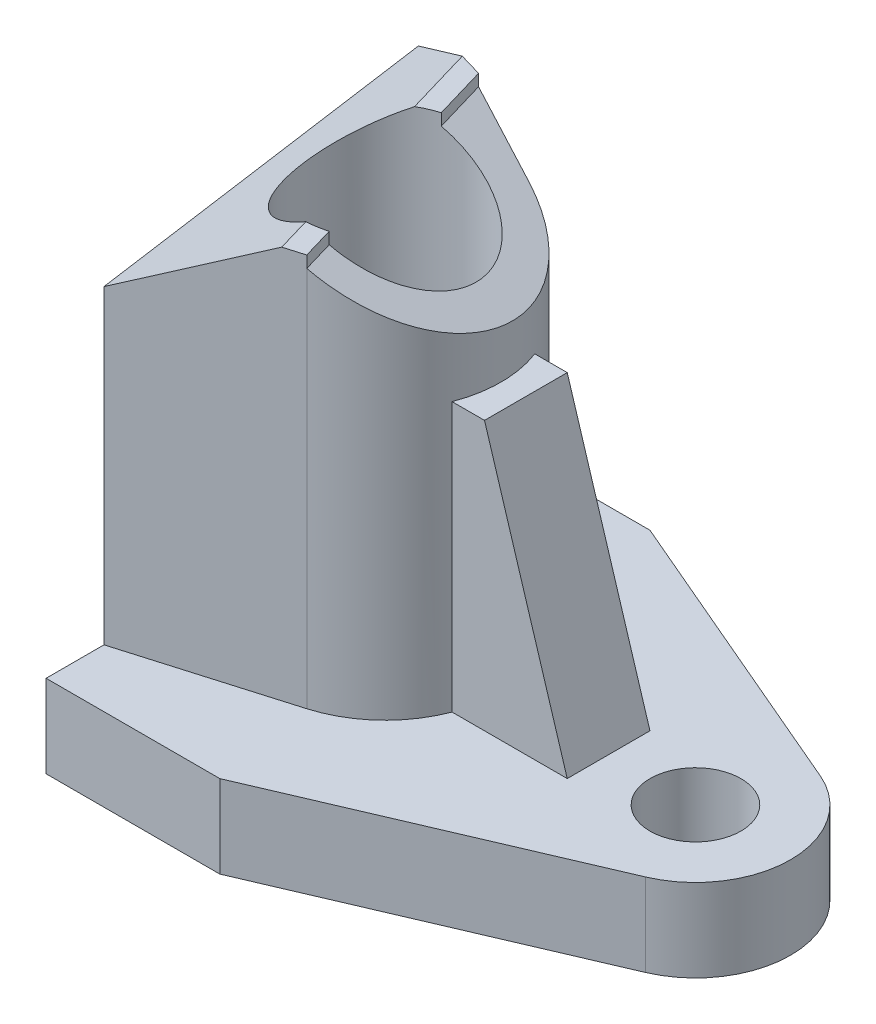
ISO-10303-21;
HEADER;
FILE_DESCRIPTION(('STEP AP214'),'2;1');
FILE_NAME('part.step','',(''),(''),'','','');
FILE_SCHEMA(('AUTOMOTIVE_DESIGN { 1 0 10303 214 1 1 1 1 }'));
ENDSEC;
DATA;
#1=APPLICATION_CONTEXT('core data for automotive mechanical design processes');
#2=APPLICATION_PROTOCOL_DEFINITION('international standard','automotive_design',2000,#1);
#3=PRODUCT_CONTEXT('',#1,'mechanical');
#4=PRODUCT('Part','Part','',(#3));
#5=PRODUCT_RELATED_PRODUCT_CATEGORY('part','',(#4));
#6=PRODUCT_DEFINITION_FORMATION('','',#4);
#7=PRODUCT_DEFINITION_CONTEXT('part definition',#1,'design');
#8=PRODUCT_DEFINITION('design','',#6,#7);
#9=PRODUCT_DEFINITION_SHAPE('','',#8);
#10=(LENGTH_UNIT() NAMED_UNIT(*) SI_UNIT(.MILLI.,.METRE.));
#11=(NAMED_UNIT(*) PLANE_ANGLE_UNIT() SI_UNIT($,.RADIAN.));
#12=(NAMED_UNIT(*) SI_UNIT($,.STERADIAN.) SOLID_ANGLE_UNIT());
#13=UNCERTAINTY_MEASURE_WITH_UNIT(LENGTH_MEASURE(1.E-05),#10,'distance_accuracy_value','');
#14=(GEOMETRIC_REPRESENTATION_CONTEXT(3) GLOBAL_UNCERTAINTY_ASSIGNED_CONTEXT((#13)) GLOBAL_UNIT_ASSIGNED_CONTEXT((#10,
#11,#12)) REPRESENTATION_CONTEXT('',''));
#15=CARTESIAN_POINT('',(0.,0.,0.));
#16=DIRECTION('',(0.,0.,1.));
#17=DIRECTION('',(1.,0.,0.));
#18=AXIS2_PLACEMENT_3D('',#15,#16,#17);
#19=CARTESIAN_POINT('',(-21.,10.,0.));
#20=DIRECTION('',(-1.,0.,0.));
#21=DIRECTION('',(0.,0.,1.));
#22=AXIS2_PLACEMENT_3D('',#19,#20,#21);
#23=PLANE('',#22);
#24=DIRECTION('',(0.,-1.,0.));
#25=VECTOR('',#24,1.);
#26=CARTESIAN_POINT('',(-21.,10.,-26.));
#27=LINE('',#26,#25);
#28=CARTESIAN_POINT('',(-21.,10.,-26.));
#29=VERTEX_POINT('',#28);
#30=CARTESIAN_POINT('',(-21.,0.,-26.));
#31=VERTEX_POINT('',#30);
#32=EDGE_CURVE('E290',#29,#31,#27,.T.);
#33=ORIENTED_EDGE('',*,*,#32,.T.);
#34=DIRECTION('',(0.,0.,-1.));
#35=VECTOR('',#34,1.);
#36=CARTESIAN_POINT('',(-21.,0.,0.));
#37=LINE('',#36,#35);
#38=CARTESIAN_POINT('',(-21.,0.,26.));
#39=VERTEX_POINT('',#38);
#40=EDGE_CURVE('E271',#39,#31,#37,.T.);
#41=ORIENTED_EDGE('',*,*,#40,.F.);
#42=DIRECTION('',(0.,-1.,0.));
#43=VECTOR('',#42,1.);
#44=CARTESIAN_POINT('',(-21.,10.,26.));
#45=LINE('',#44,#43);
#46=CARTESIAN_POINT('',(-21.,10.,26.));
#47=VERTEX_POINT('',#46);
#48=EDGE_CURVE('E312',#47,#39,#45,.T.);
#49=ORIENTED_EDGE('',*,*,#48,.F.);
#50=DIRECTION('',(0.,0.,-1.));
#51=VECTOR('',#50,1.);
#52=CARTESIAN_POINT('',(-21.,10.,0.));
#53=LINE('',#52,#51);
#54=CARTESIAN_POINT('',(-21.,10.,19.));
#55=VERTEX_POINT('',#54);
#56=EDGE_CURVE('E275',#47,#55,#53,.T.);
#57=ORIENTED_EDGE('',*,*,#56,.T.);
#58=DIRECTION('',(0.,-1.,0.));
#59=VECTOR('',#58,1.);
#60=CARTESIAN_POINT('',(-21.,57.5,19.));
#61=LINE('',#60,#59);
#62=CARTESIAN_POINT('',(-21.,47.5055162672704,19.));
#63=VERTEX_POINT('',#62);
#64=EDGE_CURVE('E252',#63,#55,#61,.T.);
#65=ORIENTED_EDGE('',*,*,#64,.F.);
#66=DIRECTION('',(0.,0.160666455096198,-0.987008758931156));
#67=VECTOR('',#66,1.);
#68=CARTESIAN_POINT('',(-21.,49.5503645251847,6.4380551930513));
#69=LINE('',#68,#67);
#70=CARTESIAN_POINT('',(-21.,53.6912012861827,-19.0000000000011));
#71=VERTEX_POINT('',#70);
#72=EDGE_CURVE('E231',#63,#71,#69,.T.);
#73=ORIENTED_EDGE('',*,*,#72,.T.);
#74=DIRECTION('',(0.,-1.,0.));
#75=VECTOR('',#74,1.);
#76=CARTESIAN_POINT('',(-21.,57.5,-19.0000000000011));
#77=LINE('',#76,#75);
#78=CARTESIAN_POINT('',(-21.,10.,-19.0000000000011));
#79=VERTEX_POINT('',#78);
#80=EDGE_CURVE('E265',#71,#79,#77,.T.);
#81=ORIENTED_EDGE('',*,*,#80,.T.);
#82=EDGE_CURVE('E277',#79,#29,#53,.T.);
#83=ORIENTED_EDGE('',*,*,#82,.T.);
#84=EDGE_LOOP('',(#33,#41,#49,#57,#65,#73,#81,#83));
#85=FACE_BOUND('',#84,.T.);
#86=ADVANCED_FACE('F45',(#85),#23,.T.);
#87=CARTESIAN_POINT('',(3.4702751003222,57.5,11.8089854095073));
#88=DIRECTION('',(-0.281945282430885,0.,-0.959430486129646));
#89=DIRECTION('',(-0.959430486129646,0.,0.281945282430885));
#90=AXIS2_PLACEMENT_3D('',#87,#88,#89);
#91=PLANE('',#90);
#92=DIRECTION('',(-0.83089117415353,-0.499999999999995,0.244171777062326));
#93=VECTOR('',#92,1.);
#94=CARTESIAN_POINT('',(-22.383250769799,46.6731264111571,19.4064922207517));
#95=LINE('',#94,#93);
#96=CARTESIAN_POINT('',(-4.39134335250773,57.5,14.1192582923178));
#97=VERTEX_POINT('',#96);
#98=EDGE_CURVE('E209',#97,#63,#95,.T.);
#99=ORIENTED_EDGE('',*,*,#98,.T.);
#100=ORIENTED_EDGE('',*,*,#64,.T.);
#101=DIRECTION('',(0.959430486129646,0.,-0.281945282430885));
#102=VECTOR('',#101,1.);
#103=CARTESIAN_POINT('',(3.4702751003222,10.,11.8089854095073));
#104=LINE('',#103,#102);
#105=CARTESIAN_POINT('',(-2.05276604596761,10.,13.432026805815));
#106=VERTEX_POINT('',#105);
#107=EDGE_CURVE('E243',#55,#106,#104,.T.);
#108=ORIENTED_EDGE('',*,*,#107,.T.);
#109=DIRECTION('',(0.,-1.,0.));
#110=VECTOR('',#109,1.);
#111=CARTESIAN_POINT('',(-2.05276604596761,57.5,13.432026805815));
#112=LINE('',#111,#110);
#113=CARTESIAN_POINT('',(-2.05276604596761,56.0927294817384,13.432026805815));
#114=VERTEX_POINT('',#113);
#115=EDGE_CURVE('E270',#114,#106,#112,.T.);
#116=ORIENTED_EDGE('',*,*,#115,.F.);
#117=CARTESIAN_POINT('',(-2.05276604596762,57.5,13.432026805815));
#118=VERTEX_POINT('',#117);
#119=EDGE_CURVE('E268',#118,#114,#112,.T.);
#120=ORIENTED_EDGE('',*,*,#119,.F.);
#121=DIRECTION('',(0.959430486129646,0.,-0.281945282430885));
#122=VECTOR('',#121,1.);
#123=CARTESIAN_POINT('',(3.4702751003222,57.5,11.8089854095073));
#124=LINE('',#123,#122);
#125=EDGE_CURVE('E242',#97,#118,#124,.T.);
#126=ORIENTED_EDGE('',*,*,#125,.F.);
#127=EDGE_LOOP('',(#99,#100,#108,#116,#120,#126));
#128=FACE_BOUND('',#127,.T.);
#129=ADVANCED_FACE('F341',(#128),#91,.F.);
#130=CARTESIAN_POINT('',(3.47027510032275,57.5,-11.8089854095068));
#131=DIRECTION('',(0.281945282430936,0.,-0.959430486129631));
#132=DIRECTION('',(-0.959430486129631,0.,-0.281945282430936));
#133=AXIS2_PLACEMENT_3D('',#130,#131,#132);
#134=PLANE('',#133);
#135=ORIENTED_EDGE('',*,*,#80,.F.);
#136=DIRECTION('',(0.863068045718996,0.436791294924048,0.253627508636911));
#137=VECTOR('',#136,1.);
#138=CARTESIAN_POINT('',(0.23751690836758,64.4393254432408,-12.7589874520087));
#139=LINE('',#138,#137);
#140=CARTESIAN_POINT('',(-13.4740888825568,57.5,-16.788380538004));
#141=VERTEX_POINT('',#140);
#142=EDGE_CURVE('E232',#71,#141,#139,.T.);
#143=ORIENTED_EDGE('',*,*,#142,.T.);
#144=DIRECTION('',(0.959430486129631,0.,0.281945282430936));
#145=VECTOR('',#144,1.);
#146=CARTESIAN_POINT('',(3.47027510032275,57.5,-11.8089854095068));
#147=LINE('',#146,#145);
#148=CARTESIAN_POINT('',(-10.6934239972705,57.5,-15.9712339518136));
#149=VERTEX_POINT('',#148);
#150=EDGE_CURVE('E250',#141,#149,#147,.T.);
#151=ORIENTED_EDGE('',*,*,#150,.T.);
#152=DIRECTION('',(0.,-1.,0.));
#153=VECTOR('',#152,1.);
#154=CARTESIAN_POINT('',(-10.6934239972705,57.5,-15.9712339518136));
#155=LINE('',#154,#153);
#156=CARTESIAN_POINT('',(-10.6934239972705,56.0927294817384,-15.9712339518136));
#157=VERTEX_POINT('',#156);
#158=EDGE_CURVE('E221',#149,#157,#155,.T.);
#159=ORIENTED_EDGE('',*,*,#158,.T.);
#160=DIRECTION('',(-0.863068045718993,0.436791294924054,-0.25362750863691));
#161=VECTOR('',#160,1.);
#162=CARTESIAN_POINT('',(0.237516908367499,50.5606745567591,-12.7589874520087));
#163=LINE('',#162,#161);
#164=CARTESIAN_POINT('',(-2.05276604596688,51.7197670087718,-13.4320268058148));
#165=VERTEX_POINT('',#164);
#166=EDGE_CURVE('E230',#165,#157,#163,.T.);
#167=ORIENTED_EDGE('',*,*,#166,.F.);
#168=DIRECTION('',(0.,-1.,0.));
#169=VECTOR('',#168,1.);
#170=CARTESIAN_POINT('',(-2.05276604596688,57.5,-13.4320268058148));
#171=LINE('',#170,#169);
#172=CARTESIAN_POINT('',(-2.05276604596688,10.,-13.4320268058148));
#173=VERTEX_POINT('',#172);
#174=EDGE_CURVE('E262',#165,#173,#171,.T.);
#175=ORIENTED_EDGE('',*,*,#174,.T.);
#176=DIRECTION('',(0.959430486129631,0.,0.281945282430936));
#177=VECTOR('',#176,1.);
#178=CARTESIAN_POINT('',(3.47027510032275,10.,-11.8089854095068));
#179=LINE('',#178,#177);
#180=EDGE_CURVE('E246',#79,#173,#179,.T.);
#181=ORIENTED_EDGE('',*,*,#180,.F.);
#182=EDGE_LOOP('',(#135,#143,#151,#159,#167,#175,#181));
#183=FACE_BOUND('',#182,.T.);
#184=ADVANCED_FACE('F348',(#183),#134,.T.);
#185=CARTESIAN_POINT('',(0.,57.5,0.));
#186=DIRECTION('',(0.,1.,0.));
#187=DIRECTION('',(0.,0.,1.));
#188=AXIS2_PLACEMENT_3D('',#185,#186,#187);
#189=PLANE('',#188);
#190=ORIENTED_EDGE('',*,*,#150,.F.);
#191=DIRECTION('',(0.281945282430885,0.,0.959430486129646));
#192=VECTOR('',#191,1.);
#193=CARTESIAN_POINT('',(-17.7837442679748,57.5,-31.4536897988404));
#194=LINE('',#193,#192);
#195=CARTESIAN_POINT('',(-11.0729926210932,57.5,-8.61769956927799));
#196=VERTEX_POINT('',#195);
#197=EDGE_CURVE('E216',#141,#196,#194,.T.);
#198=ORIENTED_EDGE('',*,*,#197,.T.);
#199=CARTESIAN_POINT('',(-6.,57.5,0.));
#200=DIRECTION('',(0.,1.,0.));
#201=DIRECTION('',(0.,0.,1.));
#202=AXIS2_PLACEMENT_3D('',#199,#200,#201);
#203=CIRCLE('',#202,10.);
#204=CARTESIAN_POINT('',(-8.81945282430885,57.5,-9.59430486129646));
#205=VERTEX_POINT('',#204);
#206=EDGE_CURVE('E240',#205,#196,#203,.T.);
#207=ORIENTED_EDGE('',*,*,#206,.F.);
#208=DIRECTION('',(0.281945282430885,0.,0.959430486129646));
#209=VECTOR('',#208,1.);
#210=CARTESIAN_POINT('',(-15.4451669614347,57.5,-32.1409212853431));
#211=LINE('',#210,#209);
#212=EDGE_CURVE('E222',#149,#205,#211,.T.);
#213=ORIENTED_EDGE('',*,*,#212,.F.);
#214=EDGE_LOOP('',(#190,#198,#207,#213));
#215=FACE_BOUND('',#214,.T.);
#216=ADVANCED_FACE('F396',(#215),#189,.T.);
#217=CARTESIAN_POINT('',(-5.60416199198704,57.5,9.99216254228345));
#218=VERTEX_POINT('',#217);
#219=CARTESIAN_POINT('',(-3.18054717569115,57.5,9.59430486129646));
#220=VERTEX_POINT('',#219);
#221=EDGE_CURVE('E245',#218,#220,#203,.T.);
#222=ORIENTED_EDGE('',*,*,#221,.F.);
#223=EDGE_CURVE('E213',#218,#97,#194,.T.);
#224=ORIENTED_EDGE('',*,*,#223,.T.);
#225=ORIENTED_EDGE('',*,*,#125,.T.);
#226=EDGE_CURVE('E225',#220,#118,#211,.T.);
#227=ORIENTED_EDGE('',*,*,#226,.F.);
#228=EDGE_LOOP('',(#222,#224,#225,#227));
#229=FACE_BOUND('',#228,.T.);
#230=ADVANCED_FACE('F389',(#229),#189,.T.);
#231=CARTESIAN_POINT('',(-6.,10.,0.));
#232=DIRECTION('',(0.,1.,0.));
#233=DIRECTION('',(0.,0.,1.));
#234=AXIS2_PLACEMENT_3D('',#231,#232,#233);
#235=CYLINDRICAL_SURFACE('',#234,10.);
#236=CARTESIAN_POINT('',(-6.,10.,0.));
#237=DIRECTION('',(0.,1.,0.));
#238=DIRECTION('',(0.,0.,1.));
#239=AXIS2_PLACEMENT_3D('',#236,#237,#238);
#240=CIRCLE('',#239,10.);
#241=CARTESIAN_POINT('',(-6.,10.,10.));
#242=VERTEX_POINT('',#241);
#243=EDGE_CURVE('E236',#242,#242,#240,.T.);
#244=ORIENTED_EDGE('',*,*,#243,.F.);
#245=EDGE_LOOP('',(#244));
#246=FACE_BOUND('',#245,.T.);
#247=CARTESIAN_POINT('',(-6.,58.9072705182616,0.));
#248=DIRECTION('',(-0.479715243064818,0.866025403784442,0.140972641215441));
#249=DIRECTION('',(0.83089117415353,0.499999999999995,-0.244171777062326));
#250=AXIS2_PLACEMENT_3D('',#247,#248,#249);
#251=ELLIPSE('',#250,11.5470053837925,10.);
#252=EDGE_CURVE('E47',#218,#196,#251,.F.);
#253=ORIENTED_EDGE('',*,*,#252,.F.);
#254=ORIENTED_EDGE('',*,*,#221,.T.);
#255=DIRECTION('',(0.,1.,0.));
#256=VECTOR('',#255,1.);
#257=CARTESIAN_POINT('',(-3.18054717569115,10.,9.59430486129646));
#258=LINE('',#257,#256);
#259=CARTESIAN_POINT('',(-3.18054717569115,56.0927294817384,9.59430486129646));
#260=VERTEX_POINT('',#259);
#261=EDGE_CURVE('E320',#260,#220,#258,.T.);
#262=ORIENTED_EDGE('',*,*,#261,.F.);
#263=CARTESIAN_POINT('',(-6.,56.0927294817384,0.));
#264=DIRECTION('',(-0.479715243064824,-0.866025403784438,0.140972641215443));
#265=DIRECTION('',(-0.830891174153526,0.500000000000001,0.244171777062325));
#266=AXIS2_PLACEMENT_3D('',#263,#264,#265);
#267=ELLIPSE('',#266,11.5470053837925,10.);
#268=CARTESIAN_POINT('',(-8.81945282430885,56.0927294817384,-9.59430486129646));
#269=VERTEX_POINT('',#268);
#270=EDGE_CURVE('E317',#260,#269,#267,.F.);
#271=ORIENTED_EDGE('',*,*,#270,.T.);
#272=DIRECTION('',(0.,1.,0.));
#273=VECTOR('',#272,1.);
#274=CARTESIAN_POINT('',(-8.81945282430885,10.,-9.59430486129646));
#275=LINE('',#274,#273);
#276=EDGE_CURVE('E325',#205,#269,#275,.F.);
#277=ORIENTED_EDGE('',*,*,#276,.F.);
#278=ORIENTED_EDGE('',*,*,#206,.T.);
#279=EDGE_LOOP('',(#253,#254,#262,#271,#277,#278));
#280=FACE_BOUND('',#279,.T.);
#281=ADVANCED_FACE('F395',(#246,#280),#235,.F.);
#282=CARTESIAN_POINT('',(0.,10.,26.));
#283=DIRECTION('',(0.,0.,-1.));
#284=DIRECTION('',(-1.,0.,0.));
#285=AXIS2_PLACEMENT_3D('',#282,#283,#284);
#286=PLANE('',#285);
#287=DIRECTION('',(1.,0.,0.));
#288=VECTOR('',#287,1.);
#289=CARTESIAN_POINT('',(0.,0.,26.));
#290=LINE('',#289,#288);
#291=CARTESIAN_POINT('',(0.,0.,26.));
#292=VERTEX_POINT('',#291);
#293=EDGE_CURVE('E288',#39,#292,#290,.T.);
#294=ORIENTED_EDGE('',*,*,#293,.T.);
#295=DIRECTION('',(0.,-1.,0.));
#296=VECTOR('',#295,1.);
#297=CARTESIAN_POINT('',(0.,10.,26.));
#298=LINE('',#297,#296);
#299=CARTESIAN_POINT('',(0.,10.,26.));
#300=VERTEX_POINT('',#299);
#301=EDGE_CURVE('E315',#300,#292,#298,.T.);
#302=ORIENTED_EDGE('',*,*,#301,.F.);
#303=DIRECTION('',(1.,0.,0.));
#304=VECTOR('',#303,1.);
#305=CARTESIAN_POINT('',(0.,10.,26.));
#306=LINE('',#305,#304);
#307=EDGE_CURVE('E274',#47,#300,#306,.T.);
#308=ORIENTED_EDGE('',*,*,#307,.F.);
#309=ORIENTED_EDGE('',*,*,#48,.T.);
#310=EDGE_LOOP('',(#294,#302,#308,#309));
#311=FACE_BOUND('',#310,.T.);
#312=ADVANCED_FACE('F368',(#311),#286,.F.);
#313=CARTESIAN_POINT('',(9.40890232991811,10.,21.9706497504953));
#314=DIRECTION('',(-0.393668654576833,0.,-0.919252408429625));
#315=DIRECTION('',(-0.919252408429625,0.,0.393668654576833));
#316=AXIS2_PLACEMENT_3D('',#313,#314,#315);
#317=PLANE('',#316);
#318=DIRECTION('',(0.919252408429625,0.,-0.393668654576833));
#319=VECTOR('',#318,1.);
#320=CARTESIAN_POINT('',(9.40890232991811,0.,21.9706497504953));
#321=LINE('',#320,#319);
#322=CARTESIAN_POINT('',(36.0271895276336,0.,10.5714026969407));
#323=VERTEX_POINT('',#322);
#324=EDGE_CURVE('E295',#292,#323,#321,.T.);
#325=ORIENTED_EDGE('',*,*,#324,.T.);
#326=DIRECTION('',(0.,-1.,0.));
#327=VECTOR('',#326,1.);
#328=CARTESIAN_POINT('',(36.0271895276336,10.,10.5714026969407));
#329=LINE('',#328,#327);
#330=CARTESIAN_POINT('',(36.0271895276336,10.,10.5714026969407));
#331=VERTEX_POINT('',#330);
#332=EDGE_CURVE('E310',#331,#323,#329,.T.);
#333=ORIENTED_EDGE('',*,*,#332,.F.);
#334=DIRECTION('',(0.919252408429625,0.,-0.393668654576833));
#335=VECTOR('',#334,1.);
#336=CARTESIAN_POINT('',(9.40890232991811,10.,21.9706497504953));
#337=LINE('',#336,#335);
#338=EDGE_CURVE('E279',#300,#331,#337,.T.);
#339=ORIENTED_EDGE('',*,*,#338,.F.);
#340=ORIENTED_EDGE('',*,*,#301,.T.);
#341=EDGE_LOOP('',(#325,#333,#339,#340));
#342=FACE_BOUND('',#341,.T.);
#343=ADVANCED_FACE('F367',(#342),#317,.F.);
#344=CARTESIAN_POINT('',(31.5,10.,0.));
#345=DIRECTION('',(0.,-1.,0.));
#346=DIRECTION('',(0.,0.,-1.));
#347=AXIS2_PLACEMENT_3D('',#344,#345,#346);
#348=CYLINDRICAL_SURFACE('',#347,11.5);
#349=CARTESIAN_POINT('',(31.5,0.,0.));
#350=DIRECTION('',(0.,1.,0.));
#351=DIRECTION('',(0.,0.,1.));
#352=AXIS2_PLACEMENT_3D('',#349,#350,#351);
#353=CIRCLE('',#352,11.5);
#354=CARTESIAN_POINT('',(36.0271895276336,0.,-10.5714026969407));
#355=VERTEX_POINT('',#354);
#356=EDGE_CURVE('E294',#323,#355,#353,.T.);
#357=ORIENTED_EDGE('',*,*,#356,.T.);
#358=DIRECTION('',(0.,-1.,0.));
#359=VECTOR('',#358,1.);
#360=CARTESIAN_POINT('',(36.0271895276336,10.,-10.5714026969407));
#361=LINE('',#360,#359);
#362=CARTESIAN_POINT('',(36.0271895276336,10.,-10.5714026969407));
#363=VERTEX_POINT('',#362);
#364=EDGE_CURVE('E307',#363,#355,#361,.T.);
#365=ORIENTED_EDGE('',*,*,#364,.F.);
#366=CARTESIAN_POINT('',(31.5,10.,0.));
#367=DIRECTION('',(0.,1.,0.));
#368=DIRECTION('',(0.,0.,1.));
#369=AXIS2_PLACEMENT_3D('',#366,#367,#368);
#370=CIRCLE('',#369,11.5);
#371=EDGE_CURVE('E278',#331,#363,#370,.T.);
#372=ORIENTED_EDGE('',*,*,#371,.F.);
#373=ORIENTED_EDGE('',*,*,#332,.T.);
#374=EDGE_LOOP('',(#357,#365,#372,#373));
#375=FACE_BOUND('',#374,.T.);
#376=ADVANCED_FACE('F410',(#375),#348,.T.);
#377=CARTESIAN_POINT('',(9.4089023299181,10.,-21.9706497504953));
#378=DIRECTION('',(0.393668654576833,0.,-0.919252408429625));
#379=DIRECTION('',(-0.919252408429625,0.,-0.393668654576833));
#380=AXIS2_PLACEMENT_3D('',#377,#378,#379);
#381=PLANE('',#380);
#382=DIRECTION('',(0.919252408429625,0.,0.393668654576833));
#383=VECTOR('',#382,1.);
#384=CARTESIAN_POINT('',(9.4089023299181,0.,-21.9706497504953));
#385=LINE('',#384,#383);
#386=CARTESIAN_POINT('',(0.,0.,-26.));
#387=VERTEX_POINT('',#386);
#388=EDGE_CURVE('E300',#387,#355,#385,.T.);
#389=ORIENTED_EDGE('',*,*,#388,.F.);
#390=DIRECTION('',(0.,-1.,0.));
#391=VECTOR('',#390,1.);
#392=CARTESIAN_POINT('',(0.,10.,-26.));
#393=LINE('',#392,#391);
#394=CARTESIAN_POINT('',(0.,10.,-26.));
#395=VERTEX_POINT('',#394);
#396=EDGE_CURVE('E303',#395,#387,#393,.T.);
#397=ORIENTED_EDGE('',*,*,#396,.F.);
#398=DIRECTION('',(0.919252408429625,0.,0.393668654576833));
#399=VECTOR('',#398,1.);
#400=CARTESIAN_POINT('',(9.4089023299181,10.,-21.9706497504953));
#401=LINE('',#400,#399);
#402=EDGE_CURVE('E285',#395,#363,#401,.T.);
#403=ORIENTED_EDGE('',*,*,#402,.T.);
#404=ORIENTED_EDGE('',*,*,#364,.T.);
#405=EDGE_LOOP('',(#389,#397,#403,#404));
#406=FACE_BOUND('',#405,.T.);
#407=ADVANCED_FACE('F403',(#406),#381,.T.);
#408=CARTESIAN_POINT('',(0.,10.,-26.));
#409=DIRECTION('',(0.,0.,-1.));
#410=DIRECTION('',(-1.,0.,0.));
#411=AXIS2_PLACEMENT_3D('',#408,#409,#410);
#412=PLANE('',#411);
#413=DIRECTION('',(1.,0.,0.));
#414=VECTOR('',#413,1.);
#415=CARTESIAN_POINT('',(0.,0.,-26.));
#416=LINE('',#415,#414);
#417=EDGE_CURVE('E297',#31,#387,#416,.T.);
#418=ORIENTED_EDGE('',*,*,#417,.F.);
#419=ORIENTED_EDGE('',*,*,#32,.F.);
#420=DIRECTION('',(1.,0.,0.));
#421=VECTOR('',#420,1.);
#422=CARTESIAN_POINT('',(0.,10.,-26.));
#423=LINE('',#422,#421);
#424=EDGE_CURVE('E282',#29,#395,#423,.T.);
#425=ORIENTED_EDGE('',*,*,#424,.T.);
#426=ORIENTED_EDGE('',*,*,#396,.T.);
#427=EDGE_LOOP('',(#418,#419,#425,#426));
#428=FACE_BOUND('',#427,.T.);
#429=ADVANCED_FACE('F356',(#428),#412,.T.);
#430=CARTESIAN_POINT('',(0.,10.,0.));
#431=DIRECTION('',(0.,1.,0.));
#432=DIRECTION('',(0.,0.,1.));
#433=AXIS2_PLACEMENT_3D('',#430,#431,#432);
#434=PLANE('',#433);
#435=DIRECTION('',(1.,0.,0.));
#436=VECTOR('',#435,1.);
#437=CARTESIAN_POINT('',(0.,10.,5.));
#438=LINE('',#437,#436);
#439=CARTESIAN_POINT('',(7.07669683062202,10.,5.));
#440=VERTEX_POINT('',#439);
#441=CARTESIAN_POINT('',(21.,10.,5.));
#442=VERTEX_POINT('',#441);
#443=EDGE_CURVE('E195',#440,#442,#438,.T.);
#444=ORIENTED_EDGE('',*,*,#443,.F.);
#445=CARTESIAN_POINT('',(-6.,10.,0.));
#446=DIRECTION('',(0.,1.,0.));
#447=DIRECTION('',(0.,0.,1.));
#448=AXIS2_PLACEMENT_3D('',#445,#446,#447);
#449=CIRCLE('',#448,14.);
#450=EDGE_CURVE('E258',#106,#440,#449,.T.);
#451=ORIENTED_EDGE('',*,*,#450,.F.);
#452=ORIENTED_EDGE('',*,*,#107,.F.);
#453=ORIENTED_EDGE('',*,*,#56,.F.);
#454=ORIENTED_EDGE('',*,*,#307,.T.);
#455=ORIENTED_EDGE('',*,*,#338,.T.);
#456=ORIENTED_EDGE('',*,*,#371,.T.);
#457=ORIENTED_EDGE('',*,*,#402,.F.);
#458=ORIENTED_EDGE('',*,*,#424,.F.);
#459=ORIENTED_EDGE('',*,*,#82,.F.);
#460=ORIENTED_EDGE('',*,*,#180,.T.);
#461=CARTESIAN_POINT('',(7.07669683062202,10.,-5.));
#462=VERTEX_POINT('',#461);
#463=EDGE_CURVE('E254',#462,#173,#449,.T.);
#464=ORIENTED_EDGE('',*,*,#463,.F.);
#465=DIRECTION('',(1.,0.,0.));
#466=VECTOR('',#465,1.);
#467=CARTESIAN_POINT('',(0.,10.,-5.));
#468=LINE('',#467,#466);
#469=CARTESIAN_POINT('',(21.,10.,-5.));
#470=VERTEX_POINT('',#469);
#471=EDGE_CURVE('E63',#462,#470,#468,.T.);
#472=ORIENTED_EDGE('',*,*,#471,.T.);
#473=DIRECTION('',(0.,0.,1.));
#474=VECTOR('',#473,1.);
#475=CARTESIAN_POINT('',(21.,10.,0.));
#476=LINE('',#475,#474);
#477=EDGE_CURVE('E57',#442,#470,#476,.F.);
#478=ORIENTED_EDGE('',*,*,#477,.F.);
#479=EDGE_LOOP('',(#444,#451,#452,#453,#454,#455,#456,#457,#458,#459,#460,#464,#472,#478));
#480=FACE_BOUND('',#479,.T.);
#481=CARTESIAN_POINT('',(31.5,10.,0.));
#482=DIRECTION('',(0.,1.,0.));
#483=DIRECTION('',(0.,0.,1.));
#484=AXIS2_PLACEMENT_3D('',#481,#482,#483);
#485=CIRCLE('',#484,5.5);
#486=CARTESIAN_POINT('',(31.5,10.,5.5));
#487=VERTEX_POINT('',#486);
#488=EDGE_CURVE('E206',#487,#487,#485,.T.);
#489=ORIENTED_EDGE('',*,*,#488,.F.);
#490=EDGE_LOOP('',(#489));
#491=FACE_BOUND('',#490,.T.);
#492=ADVANCED_FACE('F373',(#480,#491),#434,.T.);
#493=CARTESIAN_POINT('',(0.,0.,0.));
#494=DIRECTION('',(0.,1.,0.));
#495=DIRECTION('',(0.,0.,1.));
#496=AXIS2_PLACEMENT_3D('',#493,#494,#495);
#497=PLANE('',#496);
#498=CARTESIAN_POINT('',(31.5,0.,0.));
#499=DIRECTION('',(0.,1.,0.));
#500=DIRECTION('',(0.,0.,1.));
#501=AXIS2_PLACEMENT_3D('',#498,#499,#500);
#502=CIRCLE('',#501,5.5);
#503=CARTESIAN_POINT('',(31.5,0.,5.5));
#504=VERTEX_POINT('',#503);
#505=EDGE_CURVE('E207',#504,#504,#502,.T.);
#506=ORIENTED_EDGE('',*,*,#505,.T.);
#507=EDGE_LOOP('',(#506));
#508=FACE_BOUND('',#507,.T.);
#509=ORIENTED_EDGE('',*,*,#40,.T.);
#510=ORIENTED_EDGE('',*,*,#417,.T.);
#511=ORIENTED_EDGE('',*,*,#388,.T.);
#512=ORIENTED_EDGE('',*,*,#356,.F.);
#513=ORIENTED_EDGE('',*,*,#324,.F.);
#514=ORIENTED_EDGE('',*,*,#293,.F.);
#515=EDGE_LOOP('',(#509,#510,#511,#512,#513,#514));
#516=FACE_BOUND('',#515,.T.);
#517=ADVANCED_FACE('F330',(#508,#516),#497,.F.);
#518=CARTESIAN_POINT('',(-6.,57.5,0.));
#519=DIRECTION('',(0.,-1.,0.));
#520=DIRECTION('',(0.,0.,-1.));
#521=AXIS2_PLACEMENT_3D('',#518,#519,#520);
#522=CYLINDRICAL_SURFACE('',#521,14.);
#523=ORIENTED_EDGE('',*,*,#450,.T.);
#524=DIRECTION('',(0.,-1.,0.));
#525=VECTOR('',#524,1.);
#526=CARTESIAN_POINT('',(7.07669683062202,57.5,5.));
#527=LINE('',#526,#525);
#528=CARTESIAN_POINT('',(7.07669683062202,42.5,5.));
#529=VERTEX_POINT('',#528);
#530=EDGE_CURVE('E205',#440,#529,#527,.F.);
#531=ORIENTED_EDGE('',*,*,#530,.T.);
#532=CARTESIAN_POINT('',(-6.,42.5,0.));
#533=DIRECTION('',(0.,-1.,0.));
#534=DIRECTION('',(0.,0.,-1.));
#535=AXIS2_PLACEMENT_3D('',#532,#533,#534);
#536=CIRCLE('',#535,14.);
#537=CARTESIAN_POINT('',(7.07669683062202,42.5,-5.));
#538=VERTEX_POINT('',#537);
#539=EDGE_CURVE('E12',#529,#538,#536,.F.);
#540=ORIENTED_EDGE('',*,*,#539,.T.);
#541=DIRECTION('',(0.,-1.,0.));
#542=VECTOR('',#541,1.);
#543=CARTESIAN_POINT('',(7.07669683062202,57.5,-5.));
#544=LINE('',#543,#542);
#545=EDGE_CURVE('E187',#462,#538,#544,.F.);
#546=ORIENTED_EDGE('',*,*,#545,.F.);
#547=ORIENTED_EDGE('',*,*,#463,.T.);
#548=ORIENTED_EDGE('',*,*,#174,.F.);
#549=CARTESIAN_POINT('',(-6.,56.0927294817384,0.));
#550=DIRECTION('',(-0.479715243064824,-0.866025403784438,0.140972641215443));
#551=DIRECTION('',(0.830891174153526,-0.500000000000001,-0.244171777062325));
#552=AXIS2_PLACEMENT_3D('',#549,#550,#551);
#553=ELLIPSE('',#552,16.1658075373095,14.);
#554=EDGE_CURVE('E229',#165,#114,#553,.T.);
#555=ORIENTED_EDGE('',*,*,#554,.T.);
#556=ORIENTED_EDGE('',*,*,#115,.T.);
#557=EDGE_LOOP('',(#523,#531,#540,#546,#547,#548,#555,#556));
#558=FACE_BOUND('',#557,.T.);
#559=ADVANCED_FACE('F434',(#558),#522,.T.);
#560=CARTESIAN_POINT('',(-6.,10.,0.));
#561=DIRECTION('',(0.,1.,0.));
#562=DIRECTION('',(0.,0.,1.));
#563=AXIS2_PLACEMENT_3D('',#560,#561,#562);
#564=PLANE('',#563);
#565=ORIENTED_EDGE('',*,*,#243,.T.);
#566=EDGE_LOOP('',(#565));
#567=FACE_BOUND('',#566,.T.);
#568=ADVANCED_FACE('F427',(#567),#564,.T.);
#569=CARTESIAN_POINT('',(12.0005908285616,39.5768735888431,-40.2063330514901));
#570=DIRECTION('',(-0.479715243064824,-0.866025403784438,0.140972641215443));
#571=DIRECTION('',(0.874761213603876,-0.48455424791686,0.));
#572=AXIS2_PLACEMENT_3D('',#569,#570,#571);
#573=PLANE('',#572);
#574=ORIENTED_EDGE('',*,*,#554,.F.);
#575=ORIENTED_EDGE('',*,*,#166,.T.);
#576=DIRECTION('',(0.281945282430885,0.,0.959430486129646));
#577=VECTOR('',#576,1.);
#578=CARTESIAN_POINT('',(-15.4451669614346,56.0927294817384,-32.1409212853431));
#579=LINE('',#578,#577);
#580=EDGE_CURVE('E219',#157,#269,#579,.T.);
#581=ORIENTED_EDGE('',*,*,#580,.T.);
#582=ORIENTED_EDGE('',*,*,#270,.F.);
#583=EDGE_CURVE('E220',#260,#114,#579,.T.);
#584=ORIENTED_EDGE('',*,*,#583,.T.);
#585=EDGE_LOOP('',(#574,#575,#581,#582,#584));
#586=FACE_BOUND('',#585,.T.);
#587=ADVANCED_FACE('F466',(#586),#573,.F.);
#588=CARTESIAN_POINT('',(-15.4451669614347,0.,-32.1409212853431));
#589=DIRECTION('',(0.959430486129646,0.,-0.281945282430885));
#590=DIRECTION('',(-0.281945282430885,0.,-0.959430486129646));
#591=AXIS2_PLACEMENT_3D('',#588,#589,#590);
#592=PLANE('',#591);
#593=ORIENTED_EDGE('',*,*,#212,.T.);
#594=ORIENTED_EDGE('',*,*,#276,.T.);
#595=ORIENTED_EDGE('',*,*,#580,.F.);
#596=ORIENTED_EDGE('',*,*,#158,.F.);
#597=EDGE_LOOP('',(#593,#594,#595,#596));
#598=FACE_BOUND('',#597,.T.);
#599=ADVANCED_FACE('F471',(#598),#592,.T.);
#600=ORIENTED_EDGE('',*,*,#261,.T.);
#601=ORIENTED_EDGE('',*,*,#226,.T.);
#602=ORIENTED_EDGE('',*,*,#119,.T.);
#603=ORIENTED_EDGE('',*,*,#583,.F.);
#604=EDGE_LOOP('',(#600,#601,#602,#603));
#605=FACE_BOUND('',#604,.T.);
#606=ADVANCED_FACE('F342',(#605),#592,.T.);
#607=CARTESIAN_POINT('',(-35.775651685266,46.6731264111571,-26.1664558704065));
#608=DIRECTION('',(-0.479715243064818,0.866025403784442,0.140972641215441));
#609=DIRECTION('',(-0.874761213603879,-0.484554247916854,0.));
#610=AXIS2_PLACEMENT_3D('',#607,#608,#609);
#611=PLANE('',#610);
#612=ORIENTED_EDGE('',*,*,#98,.F.);
#613=ORIENTED_EDGE('',*,*,#223,.F.);
#614=ORIENTED_EDGE('',*,*,#252,.T.);
#615=ORIENTED_EDGE('',*,*,#197,.F.);
#616=ORIENTED_EDGE('',*,*,#142,.F.);
#617=ORIENTED_EDGE('',*,*,#72,.F.);
#618=EDGE_LOOP('',(#612,#613,#614,#615,#616,#617));
#619=FACE_BOUND('',#618,.T.);
#620=ADVANCED_FACE('F335',(#619),#611,.T.);
#621=CARTESIAN_POINT('',(31.5,-37.5,0.));
#622=DIRECTION('',(0.,1.,0.));
#623=DIRECTION('',(0.,0.,1.));
#624=AXIS2_PLACEMENT_3D('',#621,#622,#623);
#625=CYLINDRICAL_SURFACE('',#624,5.5);
#626=ORIENTED_EDGE('',*,*,#488,.T.);
#627=EDGE_LOOP('',(#626));
#628=FACE_BOUND('',#627,.T.);
#629=ORIENTED_EDGE('',*,*,#505,.F.);
#630=EDGE_LOOP('',(#629));
#631=FACE_BOUND('',#630,.T.);
#632=ADVANCED_FACE('F329',(#628,#631),#625,.F.);
#633=CARTESIAN_POINT('',(8.,42.5,0.));
#634=DIRECTION('',(0.,-1.,0.));
#635=DIRECTION('',(1.,0.,0.));
#636=AXIS2_PLACEMENT_3D('',#633,#634,#635);
#637=PLANE('',#636);
#638=ORIENTED_EDGE('',*,*,#539,.F.);
#639=DIRECTION('',(1.,0.,0.));
#640=VECTOR('',#639,1.);
#641=CARTESIAN_POINT('',(11.,42.5,5.));
#642=LINE('',#641,#640);
#643=CARTESIAN_POINT('',(11.,42.5,5.));
#644=VERTEX_POINT('',#643);
#645=EDGE_CURVE('E174',#529,#644,#642,.T.);
#646=ORIENTED_EDGE('',*,*,#645,.T.);
#647=DIRECTION('',(0.,0.,1.));
#648=VECTOR('',#647,1.);
#649=CARTESIAN_POINT('',(11.,42.5,0.));
#650=LINE('',#649,#648);
#651=CARTESIAN_POINT('',(11.,42.5,-5.));
#652=VERTEX_POINT('',#651);
#653=EDGE_CURVE('E180',#652,#644,#650,.T.);
#654=ORIENTED_EDGE('',*,*,#653,.F.);
#655=DIRECTION('',(1.,0.,0.));
#656=VECTOR('',#655,1.);
#657=CARTESIAN_POINT('',(11.,42.5,-5.));
#658=LINE('',#657,#656);
#659=EDGE_CURVE('E197',#538,#652,#658,.T.);
#660=ORIENTED_EDGE('',*,*,#659,.F.);
#661=EDGE_LOOP('',(#638,#646,#654,#660));
#662=FACE_BOUND('',#661,.T.);
#663=ADVANCED_FACE('F177',(#662),#637,.F.);
#664=CARTESIAN_POINT('',(11.,42.5,0.));
#665=DIRECTION('',(-0.95577900872195,-0.294085848837523,0.));
#666=DIRECTION('',(0.294085848837523,-0.95577900872195,0.));
#667=AXIS2_PLACEMENT_3D('',#664,#665,#666);
#668=PLANE('',#667);
#669=DIRECTION('',(0.294085848837523,-0.95577900872195,0.));
#670=VECTOR('',#669,1.);
#671=CARTESIAN_POINT('',(11.,42.5,5.));
#672=LINE('',#671,#670);
#673=EDGE_CURVE('E181',#644,#442,#672,.T.);
#674=ORIENTED_EDGE('',*,*,#673,.T.);
#675=ORIENTED_EDGE('',*,*,#477,.T.);
#676=DIRECTION('',(0.294085848837523,-0.95577900872195,0.));
#677=VECTOR('',#676,1.);
#678=CARTESIAN_POINT('',(11.,42.5,-5.));
#679=LINE('',#678,#677);
#680=EDGE_CURVE('E184',#652,#470,#679,.T.);
#681=ORIENTED_EDGE('',*,*,#680,.F.);
#682=ORIENTED_EDGE('',*,*,#653,.T.);
#683=EDGE_LOOP('',(#674,#675,#681,#682));
#684=FACE_BOUND('',#683,.T.);
#685=ADVANCED_FACE('F186',(#684),#668,.F.);
#686=CARTESIAN_POINT('',(11.,28.75,5.));
#687=DIRECTION('',(0.,0.,1.));
#688=DIRECTION('',(1.,0.,0.));
#689=AXIS2_PLACEMENT_3D('',#686,#687,#688);
#690=PLANE('',#689);
#691=ORIENTED_EDGE('',*,*,#530,.F.);
#692=ORIENTED_EDGE('',*,*,#443,.T.);
#693=ORIENTED_EDGE('',*,*,#673,.F.);
#694=ORIENTED_EDGE('',*,*,#645,.F.);
#695=EDGE_LOOP('',(#691,#692,#693,#694));
#696=FACE_BOUND('',#695,.T.);
#697=ADVANCED_FACE('F194',(#696),#690,.T.);
#698=CARTESIAN_POINT('',(11.,28.75,-5.));
#699=DIRECTION('',(0.,0.,1.));
#700=DIRECTION('',(1.,0.,0.));
#701=AXIS2_PLACEMENT_3D('',#698,#699,#700);
#702=PLANE('',#701);
#703=ORIENTED_EDGE('',*,*,#471,.F.);
#704=ORIENTED_EDGE('',*,*,#545,.T.);
#705=ORIENTED_EDGE('',*,*,#659,.T.);
#706=ORIENTED_EDGE('',*,*,#680,.T.);
#707=EDGE_LOOP('',(#703,#704,#705,#706));
#708=FACE_BOUND('',#707,.T.);
#709=ADVANCED_FACE('F521',(#708),#702,.F.);
#710=CLOSED_SHELL('',(#86,#129,#184,#216,#230,#281,#312,#343,#376,#407,#429,#492,#517,#559,#568,
#587,#599,#606,#620,#632,#663,#685,#697,#709));
#711=MANIFOLD_SOLID_BREP('B2',#710);
#712=ADVANCED_BREP_SHAPE_REPRESENTATION('',(#18,#711),#14);
#713=SHAPE_DEFINITION_REPRESENTATION(#9,#712);
ENDSEC;
END-ISO-10303-21;
